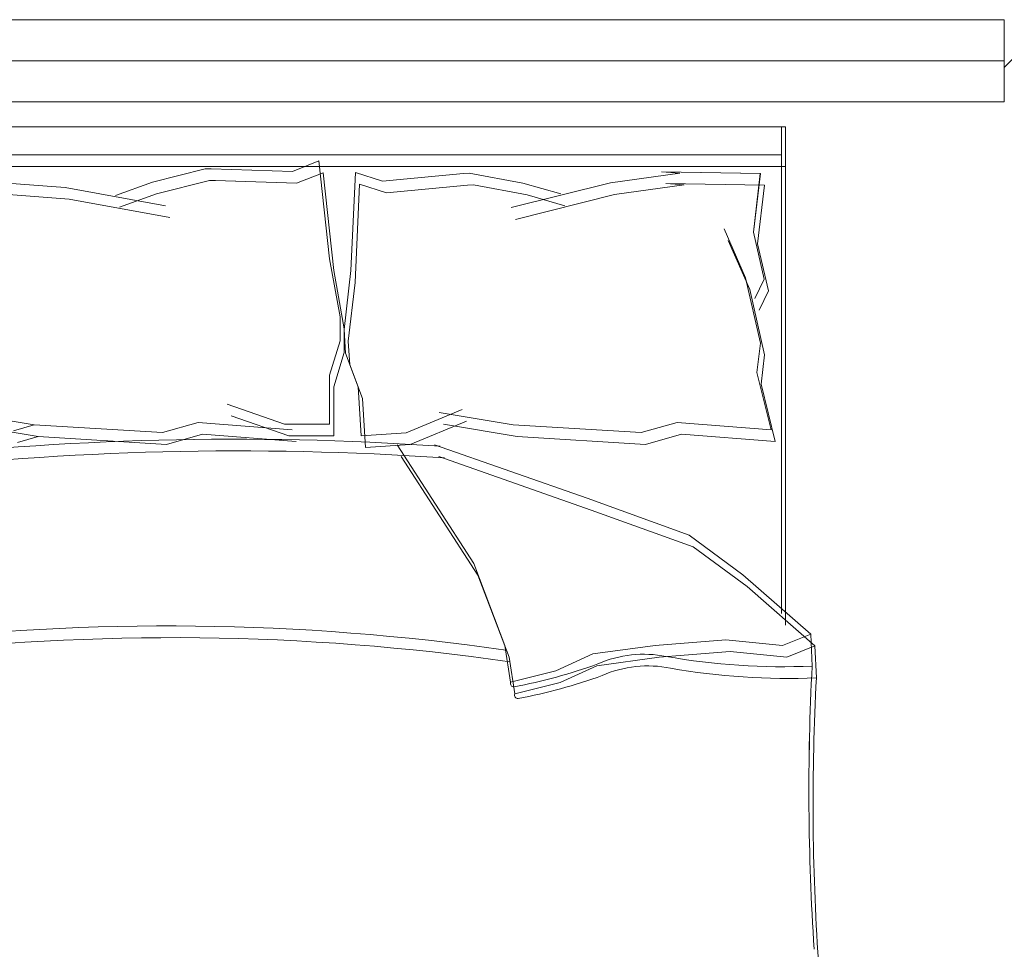
# Model space of a CAD drawing. Units: inches. Extents: x 1885 to 2748, y 783 to 2421.
# Tile 99 of 117: x 2395 to 2449, y 2302 to 2353. Entities that reach past the tile are written whole.
import ezdxf

# ---------------------------------------------------------------- set-up
doc = ezdxf.new("R2010")
doc.units = ezdxf.units.IN
doc.layers.add('A-FURN', color=8, linetype='Continuous', lineweight=13)
doc.layers.add('A-GLAZ', color=181, linetype='Continuous', lineweight=18)
doc.layers.add('A-WALL-PATT', color=85, linetype='Continuous', lineweight=13, true_color=0x58ba48)

# ---------------------------------------------------------------- blocks, each defined once
blk = doc.blocks.new('BED-DOUBLE')
for p, q in [((27.749, 52.866), (24.499, 49.161)), ((27.75, 52.866), (24.499, 49.161)), ((28.389, 53.095), (25.139, 49.389)), ((28.389, 53.094), (25.139, 49.389)), ((29.494, 52.946), (27.749, 52.866, 3.871)), ((28.369, 51.329), (27.749, 52.866)), ((29.494, 52.945), (27.75, 52.866, 3.871)), ((28.369, 51.329), (27.75, 52.866)), ((30.133, 53.174), (28.389, 53.095, 3.871)), ((30.133, 53.174), (28.389, 53.094, 3.871)), ((29.008, 51.558), (28.389, 53.095)), ((29.008, 51.557), (28.389, 53.094)), ((0.004, 51.493), (0.643, 51.492)), ((0.004, 3.474), (0.004, 51.493)), ((0.004, 51.264), (26.614, 51.264)), ((0.004, 51.264), (26.614, 51.264)), ((0.643, 51.493), (27.253, 51.493)), ((0.643, 51.492), (27.253, 51.492)), ((1.537, 3.474), (1.537, 51.264)), ((1.537, 3.474), (1.537, 51.264)), ((2.177, 3.702), (2.177, 51.493)), ((2.177, 3.702), (2.177, 51.492)), ((28.059, 48.232), (28.369, 51.329)), ((28.059, 48.231), (28.369, 51.329)), ((28.698, 48.46), (29.008, 51.558)), ((28.698, 48.46), (29.008, 51.557)), ((16.576, 50.697), (13.438, 49.922)), ((16.576, 50.697), (13.438, 49.921)), ((17.216, 50.925), (14.077, 50.15)), ((17.216, 50.925), (14.077, 50.15)), ((16.173, 45.565), (16.576, 50.697)), ((16.173, 45.565), (16.576, 50.697)), ((16.812, 45.794), (17.216, 50.925)), ((16.812, 45.793), (17.216, 50.925)), ((2.561, 50.111), (2.464, 44.708)), ((2.561, 50.11), (2.464, 44.708)), ((2.561, 50.111), (5.771, 49.732)), ((2.561, 50.11), (5.771, 49.732)), ((3.2, 50.339), (3.103, 44.937)), ((3.2, 50.339), (3.103, 44.936)), ((3.2, 50.339), (6.411, 49.96)), ((3.2, 50.339), (6.411, 49.96)), ((5.771, 49.732), (8.342, 50.327)), ((5.771, 49.732), (8.342, 50.327)), ((6.411, 49.96), (8.981, 50.556)), ((6.411, 49.96), (8.981, 50.555)), ((11.832, 50.111), (8.261, 49.308)), ((11.832, 50.111), (8.261, 49.308)), ((8.342, 50.327), (9.388, 49.813)), ((8.342, 50.327), (9.388, 49.813)), ((12.472, 50.339), (8.9, 49.537)), ((12.472, 50.339), (8.9, 49.536)), ((8.981, 50.556), (10.027, 50.042)), ((8.981, 50.555), (10.027, 50.041)), ((13.438, 49.922), (11.832, 50.111)), ((13.438, 49.921), (11.832, 50.111)), ((14.077, 50.15), (12.472, 50.339)), ((14.077, 50.15), (12.472, 50.339)), ((8.9, 49.537), (6.221, 48.355)), ((8.9, 49.536), (6.221, 48.355)), ((8.261, 49.308), (5.582, 48.127)), ((8.261, 49.308), (5.582, 48.127)), ((24.499, 49.161), (22.332, 46.218)), ((24.499, 49.161), (22.332, 46.218)), ((25.139, 49.389), (22.972, 46.447)), ((25.139, 49.389), (22.972, 46.447)), ((29.008, 44.588), (28.698, 48.46)), ((29.008, 44.588), (28.698, 48.46)), ((28.369, 44.36), (28.059, 48.232)), ((28.369, 44.36), (28.059, 48.231)), ((22.972, 46.447), (20.96, 40.871)), ((22.972, 46.447), (20.96, 40.871)), ((3.103, 44.937), (3.185, 45.939)), ((3.103, 44.936), (3.185, 45.939)), ((3.185, 45.939), (3.712, 42.141)), ((3.185, 45.939), (3.712, 42.141)), ((17.369, 43.833), (16.812, 45.794)), ((17.369, 43.833), (16.812, 45.793)), ((22.332, 46.218), (20.32, 40.643)), ((22.332, 46.218), (20.32, 40.643)), ((2.464, 44.708), (2.546, 45.711)), ((2.464, 44.708), (2.546, 45.711)), ((2.546, 45.711), (3.073, 41.913)), ((2.546, 45.711), (3.073, 41.913)), ((16.73, 43.605), (16.173, 45.565)), ((16.73, 43.605), (16.173, 45.565)), ((28.833, 40.953), (28.369, 44.36)), ((28.833, 40.952), (28.369, 44.36)), ((29.472, 41.181), (29.008, 44.588)), ((29.472, 41.181), (29.008, 44.588)), ((16.299, 36.595), (16.73, 43.605)), ((16.299, 36.595), (16.73, 43.605)), ((16.938, 36.823), (17.369, 43.833)), ((16.938, 36.823), (17.369, 43.833)), ((3.712, 42.141), (5.065, 36.722)), ((3.712, 42.141), (5.065, 36.722)), ((3.073, 41.913), (4.426, 36.494)), ((3.073, 41.913), (4.426, 36.493)), ((29.762, 38.939), (28.833, 40.953)), ((29.762, 38.939), (28.833, 40.952)), ((30.401, 39.168), (29.472, 41.181)), ((30.401, 39.167), (29.472, 41.181)), ((20.32, 40.643), (17.387, 32.305)), ((20.32, 40.643), (17.387, 32.305)), ((20.96, 40.871), (18.026, 32.533)), ((20.96, 40.871), (18.026, 32.533)), ((4.317, 39.427), (3.721, 37.362)), ((4.317, 39.427), (3.721, 37.362)), ((3.677, 39.199), (3.082, 37.134)), ((3.677, 39.199), (3.082, 37.134)), ((30.381, 36.461), (29.762, 38.939)), ((30.381, 36.461), (29.762, 38.939)), ((31.02, 36.69), (30.401, 39.168)), ((31.02, 36.689), (30.401, 39.167)), ((3.721, 37.362), (3.18, 34.432)), ((3.721, 37.362), (3.18, 34.431)), ((3.082, 37.134), (2.541, 34.203)), ((3.082, 37.134), (2.541, 34.203)), ((16.271, 32.791), (16.938, 36.823)), ((16.272, 32.791), (16.938, 36.823)), ((29.008, 36.38), (31.02, 36.69)), ((29.008, 36.38), (31.02, 36.689)), ((15.632, 32.563), (16.299, 36.595)), ((15.632, 32.563), (16.299, 36.595)), ((23.88, 34.448), (28.369, 36.152)), ((23.88, 34.448), (28.369, 36.151)), ((24.519, 34.676), (29.008, 36.38)), ((24.519, 34.676), (29.008, 36.38)), ((28.369, 36.152), (30.381, 36.461)), ((28.369, 36.151), (30.381, 36.461)), ((17.387, 30.258), (23.88, 34.448)), ((17.387, 30.258), (23.88, 34.448)), ((18.026, 30.486), (24.519, 34.676)), ((18.026, 30.486), (24.519, 34.676)), ((2.541, 34.203), (2.561, 33.882)), ((2.541, 34.203), (2.561, 33.882)), ((3.18, 34.432), (3.2, 34.111)), ((3.18, 34.431), (3.2, 34.11)), ((3.2, 34.111), (3.622, 29.683)), ((3.2, 34.11), (3.622, 29.683)), ((17.382, 30.977), (16.097, 34.048)), ((17.382, 30.977), (16.097, 34.048)), ((2.561, 33.882), (2.982, 29.454)), ((2.561, 33.882), (2.982, 29.454)), ((16.743, 30.749), (15.458, 33.819)), ((16.743, 30.749), (15.458, 33.819)), ((16.896, 28.296), (16.743, 30.749)), ((16.896, 28.296), (16.743, 30.749)), ((17.536, 28.525), (17.382, 30.977)), ((17.536, 28.524), (17.382, 30.977)), ((3.622, 29.683), (3.135, 28.204)), ((3.622, 29.683), (3.135, 28.204)), ((2.982, 29.454), (2.495, 27.976)), ((2.982, 29.454), (2.495, 27.975)), ((3.135, 28.204), (8.51, 27.961)), ((3.135, 28.204), (8.51, 27.96)), ((12.38, 27.435), (14.22, 28.129)), ((12.38, 27.434), (14.22, 28.129)), ((13.02, 27.663), (14.86, 28.357)), ((13.02, 27.663), (14.86, 28.357)), ((14.22, 28.129), (16.896, 28.296)), ((14.22, 28.129), (16.896, 28.296)), ((14.86, 28.357), (17.536, 28.525)), ((14.86, 28.357), (17.536, 28.524)), ((2.495, 27.976), (7.871, 27.732)), ((2.495, 27.975), (7.871, 27.732)), ((7.871, 27.732), (11.082, 27.354)), ((7.871, 27.732), (11.082, 27.353)), ((8.51, 27.961), (11.721, 27.582)), ((8.51, 27.96), (11.721, 27.582)), ((11.721, 27.582), (13.02, 27.663)), ((11.721, 27.582), (13.02, 27.663)), ((7.224, 26.56), (10.404, 27.138)), ((7.224, 26.559), (10.405, 27.137)), ((7.863, 26.788), (11.044, 27.366)), ((7.863, 26.788), (11.044, 27.366)), ((10.404, 27.138), (11.706, 27.138)), ((10.405, 27.137), (11.706, 27.137)), ((11.044, 27.366), (12.345, 27.366)), ((11.044, 27.366), (12.345, 27.366)), ((11.082, 27.354), (12.38, 27.435)), ((11.082, 27.353), (12.38, 27.434)), ((11.706, 27.138), (13.585, 26.56)), ((11.706, 27.137), (13.585, 26.559)), ((12.345, 27.366), (14.225, 26.788)), ((12.345, 27.366), (14.225, 26.788)), ((1.874, 25.981), (7.224, 26.56)), ((1.874, 25.981), (7.224, 26.559)), ((2.513, 26.21), (7.863, 26.788)), ((2.513, 26.209), (7.863, 26.788)), ((13.585, 26.56), (16.267, 26.56)), ((13.585, 26.559), (16.267, 26.559)), ((14.225, 26.788), (16.906, 26.788)), ((14.225, 26.788), (16.906, 26.788)), ((16.267, 26.56), (16.267, 24.102)), ((16.267, 26.559), (16.267, 24.102)), ((16.906, 26.788), (16.906, 24.33)), ((16.906, 26.788), (16.906, 24.33)), ((2.452, 24.536), (1.874, 25.981)), ((2.452, 24.535), (1.874, 25.981)), ((3.091, 24.764), (2.513, 26.21)), ((3.091, 24.764), (2.513, 26.209)), ((2.947, 20.319), (3.091, 24.764)), ((2.947, 20.318), (3.091, 24.764)), ((2.308, 20.09), (2.452, 24.536)), ((2.308, 20.09), (2.452, 24.535)), ((16.906, 24.33), (15.815, 21.186)), ((16.906, 24.33), (15.815, 21.186)), ((16.173, 19.383), (16.576, 24.515)), ((16.173, 19.382), (16.576, 24.514)), ((16.812, 19.611), (17.216, 24.743)), ((16.812, 19.611), (17.216, 24.743)), ((16.267, 24.102), (15.176, 20.957)), ((16.267, 24.102), (15.176, 20.957)), ((2.308, 19.769), (2.308, 20.09)), ((2.308, 19.768), (2.308, 20.09)), ((2.947, 19.997), (2.947, 20.319)), ((2.947, 19.997), (2.947, 20.318)), ((3.67, 17.106), (2.947, 19.997)), ((3.67, 17.105), (2.947, 19.997)), ((3.031, 16.877), (2.308, 19.769)), ((3.031, 16.877), (2.308, 19.768)), ((16.73, 17.422), (16.173, 19.383)), ((16.73, 17.422), (16.173, 19.382)), ((17.369, 17.651), (16.812, 19.611)), ((17.369, 17.65), (16.812, 19.611)), ((3.959, 12.335), (4.971, 17.829)), ((3.959, 12.335), (4.971, 17.828)), ((3.32, 12.107), (4.332, 17.6)), ((3.32, 12.107), (4.332, 17.6)), ((16.299, 10.412), (16.73, 17.422)), ((16.299, 10.412), (16.73, 17.422)), ((16.938, 10.641), (17.369, 17.651)), ((16.938, 10.64), (17.369, 17.65)), ((3.753, 14.854), (3.031, 16.877)), ((3.753, 14.853), (3.031, 16.877)), ((4.393, 15.082), (3.67, 17.106)), ((4.393, 15.082), (3.67, 17.105)), ((3.031, 8.284), (3.32, 12.107)), ((3.031, 8.283), (3.32, 12.107)), ((3.67, 8.512), (3.959, 12.335)), ((3.67, 8.512), (3.959, 12.335)), ((15.632, 6.38), (16.299, 10.412)), ((15.632, 6.38), (16.299, 10.412)), ((16.271, 6.609), (16.938, 10.641)), ((16.272, 6.609), (16.938, 10.64)), ((16.299, 10.412), (16.622, 9.279)), ((16.299, 10.412), (16.622, 9.279)), ((16.938, 10.641), (17.261, 9.508)), ((16.938, 10.64), (17.261, 9.507))]:
    blk.add_line(p, q)
for centre, radius, start, end in [((-6.653, 51.326), 36.183, 349.8763, 2.5657), ((-6.653, 51.326), 36.183, 349.8763, 2.5657), ((36.319, 182.265), 129.499, 266.97912, 273.83645), ((36.319, 182.264), 129.499, 266.97912, 273.83645), ((-6.013, 51.554), 36.183, 349.8763, 2.5657), ((-6.013, 51.554), 36.183, 349.8763, 2.5657), ((36.958, 182.493), 129.499, 266.97912, 273.83645), ((36.958, 182.493), 129.499, 266.97912, 273.83645), ((35.07, 43.742), 6.224, 168.6608, 203.7384), ((35.07, 43.742), 6.224, 168.6608, 203.7384), ((35.709, 43.971), 6.224, 168.6608, 203.7384), ((35.709, 43.97), 6.224, 168.6608, 203.7384), ((2.125, 31.381), 29.654, 10.6617, 19.8806), ((2.125, 31.381), 29.654, 10.6617, 19.8806), ((1.486, 31.152), 29.654, 10.6617, 19.8806), ((1.486, 31.152), 29.654, 10.6617, 19.8806), ((30.443, 36.635), 0.185, 250.2464, 1.1377), ((30.443, 36.635), 0.185, 250.2464, 1.1377), ((31.082, 36.863), 0.185, 250.2464, 1.1377), ((31.082, 36.863), 0.185, 250.2464, 1.1377), ((156.32, 17.754), 129.02, 171.78449, 186.90062), ((156.32, 17.754), 129.02, 171.78449, 186.90062), ((156.959, 17.983), 129.02, 171.78449, 186.90062), ((156.959, 17.983), 129.02, 171.78449, 186.90062), ((182.695, 21.586), 164.969, 176.08655, 186.78213), ((182.695, 21.586), 164.969, 176.08655, 186.78213), ((182.056, 21.358), 164.969, 176.08655, 186.78213), ((182.056, 21.357), 164.969, 176.08655, 186.78213)]:
    blk.add_arc(centre, radius, start, end)
blk = doc.blocks.new('WIN-60')
for p, q in [((0.004, 59.998), (4.504, 59.998)), ((0.004, 59.998), (0.004, -0.002)), ((4.504, 59.998), (2.254, 59.998)), ((2.254, 59.998), (2.254, -0.002)), ((4.504, -0.002), (4.504, 59.998))]:
    blk.add_line(p, q)

msp = doc.modelspace()

# ---------------------------------------------------------------- hatches: boundary and pattern name
at = {"layer": 'A-WALL-PATT'}
h = msp.add_hatch(dxfattribs=at)
h.set_pattern_fill('ANSI32', color=256)
h.paths.add_polyline_path([(2007.772, 2318.006), (1980.774, 2318.006), (1980.774, 2281.215), (1985.274, 2281.215), (1985.274, 2313.506), (2007.772, 2313.506), (2007.772, 2315.756)])
h.paths.add_polyline_path([(2094.324, 2318.006), (2067.772, 2318.006), (2067.772, 2313.506), (2094.324, 2313.506), (2094.324, 2315.756)])
h.paths.add_polyline_path([(2131.367, 2315.756), (2131.367, 2318.006), (2131.189, 2318.006), (2112.609, 2318.006), (2112.609, 2313.506), (2117.274, 2313.506), (2117.274, 2255.201), (2121.774, 2255.201), (2121.774, 2313.506), (2131.367, 2313.506)])
h.paths.add_polyline_path([(2190.512, 2318.006), (2155.367, 2318.006), (2155.367, 2313.506), (2169.774, 2313.506), (2169.774, 2229.506), (2121.774, 2229.506), (2121.774, 2233.451), (2119.524, 2233.451), (2117.274, 2233.451), (2117.274, 2201.101), (2121.774, 2201.101), (2121.774, 2225.006), (2169.774, 2225.006), (2169.774, 2165.006), (2306.274, 2165.006), (2306.274, 2066.006), (2310.774, 2066.006), (2344.274, 2066.006), (2486.274, 2066.006), (2486.274, 1886.006), (2483.02, 1886.006), (2483.02, 1881.506), (2486.274, 1881.506), (2486.274, 1880.678), (2490.774, 1880.678), (2490.774, 2070.506), (2344.274, 2070.506), (2310.774, 2070.506), (2310.774, 2165.006), (2310.774, 2173.636), (2308.524, 2173.636), (2306.274, 2173.636), (2306.274, 2169.506), (2174.274, 2169.506), (2174.274, 2313.506), (2190.512, 2313.506), (2190.512, 2315.756)])
h.paths.add_polyline_path([(1985.274, 2221.215), (1980.774, 2221.215), (1980.774, 2165.006), (1992.774, 2165.006), (1992.774, 2141.927), (1997.274, 2141.927), (1997.274, 2165.006), (2117.274, 2165.006), (2117.274, 2163.126), (2121.774, 2163.126), (2121.774, 2172.734), (2119.524, 2172.734), (2117.274, 2172.734), (2117.274, 2169.506), (1985.274, 2169.506)])
h.paths.add_polyline_path([(1997.274, 2105.927), (1992.774, 2105.927), (1992.774, 2070.506), (2016.774, 2070.506), (2016.774, 2059.123), (2019.024, 2059.123), (2021.274, 2059.123), (2021.274, 2070.506), (2117.274, 2070.506), (2117.274, 2022.506), (2114.423, 2022.506), (2114.423, 2018.006), (2123.627, 2018.006), (2123.627, 2020.256), (2123.627, 2022.506), (2121.774, 2022.506), (2121.774, 2142.587), (2119.524, 2142.587), (2117.274, 2142.587), (2117.274, 2075.006), (1997.274, 2075.006)])
h.paths.add_polyline_path([(2092.029, 2020.256), (2092.029, 2022.506), (2021.274, 2022.506), (2021.274, 2035.123), (2016.774, 2035.123), (2016.774, 2018.006), (2016.774, 1978.784), (2021.274, 1978.784), (2021.274, 2018.006), (2092.029, 2018.006)])
h.paths.add_polyline_path([(2260.938, 2022.506), (2153.105, 2022.506), (2153.105, 2020.256), (2153.105, 2018.006), (2155.274, 2018.006), (2155.274, 1886.006), (2107.629, 1886.006), (2107.629, 1881.506), (2182.911, 1881.506), (2182.911, 1883.756), (2182.911, 1886.006), (2159.774, 1886.006), (2159.774, 2018.006), (2260.938, 2018.006), (2260.938, 2020.256)])
h.paths.add_polyline_path([(2047.629, 1883.756), (2047.629, 1886.006), (2021.274, 1886.006), (2021.274, 1918.784), (2019.024, 1918.784), (2016.774, 1918.784), (2016.774, 1881.506), (2047.629, 1881.506)])
h.paths.add_polyline_path([(2306.361, 1883.756), (2306.361, 1886.006), (2296.274, 1886.006), (2296.274, 1982.006), (2316.535, 1982.006), (2316.535, 1984.256), (2316.535, 1986.506), (2296.274, 1986.506), (2296.274, 2022.506), (2289.276, 2022.506), (2289.276, 2018.006), (2291.774, 2018.006), (2291.774, 1886.006), (2242.911, 1886.006), (2242.911, 1881.506), (2306.361, 1881.506)], flags=17)
h.paths.add_polyline_path([(1985.274, 1843.006), (2021.6, 1843.006), (2021.534, 1845.441), (2021.477, 1847.506), (1980.774, 1847.506), (1980.774, 1809.446), (1985.274, 1809.446)])
h.paths.add_polyline_path([(2131.482, 1845.256), (2131.482, 1847.506), (2081.534, 1847.506), (2081.534, 1843.006), (2117.274, 1843.006), (2117.274, 1784.147), (2119.524, 1784.147), (2121.774, 1784.147), (2121.774, 1843.006), (2131.482, 1843.006)])
h.paths.add_polyline_path([(2203.886, 1847.506), (2155.482, 1847.506), (2155.482, 1843.006), (2169.774, 1843.006), (2169.774, 1759.006), (2121.774, 1759.006), (2121.774, 1761.457), (2117.274, 1761.457), (2117.274, 1730.429), (2121.774, 1730.429), (2121.774, 1754.506), (2177.421, 1754.506), (2177.421, 1756.756), (2177.421, 1759.006), (2174.274, 1759.006), (2174.274, 1843.006), (2203.886, 1843.006)])
h.paths.add_polyline_path([(2335.554, 1845.256), (2335.554, 1847.506), (2239.886, 1847.506), (2239.886, 1843.006), (2306.274, 1843.006), (2306.274, 1759.006), (2199.486, 1759.006), (2199.486, 1754.506), (2310.774, 1754.506), (2310.774, 1843.006), (2335.554, 1843.006)])
h.paths.add_polyline_path([(2348.774, 2022.506), (2344.274, 2022.506), (2344.274, 1986.506), (2341.681, 1986.506), (2341.681, 1982.006), (2344.274, 1982.006), (2344.274, 1886.006), (2330.361, 1886.006), (2330.361, 1881.506), (2361.627, 1881.506), (2361.627, 1883.756), (2361.627, 1886.006), (2348.774, 1886.006)], flags=17)
h.paths.add_polyline_path([(2283.251, 2315.756), (2283.251, 2318.006), (2238.512, 2318.006), (2238.512, 2313.506), (2283.251, 2313.506)], flags=17)
h.paths.add_polyline_path([(2363.274, 2348.006), (2388.677, 2348.006), (2388.677, 2350.256), (2388.677, 2352.506), (2358.774, 2352.506), (2358.774, 2348.006), (2358.774, 2318.006), (2344.481, 2318.006), (2344.481, 2313.506), (2358.774, 2313.506), (2358.774, 2229.506), (2310.774, 2229.506), (2310.774, 2231.952), (2306.274, 2231.952), (2306.274, 2205.611), (2310.774, 2205.611), (2310.774, 2225.006), (2358.774, 2225.006), (2358.774, 2211.506), (2452.329, 2211.506), (2452.329, 2213.756), (2452.329, 2216.006), (2363.274, 2216.006), (2363.274, 2318.006)])
h.paths.add_polyline_path([(2310.774, 2313.506), (2320.481, 2313.506), (2320.481, 2315.756), (2320.481, 2318.006), (2302.728, 2318.006), (2302.728, 2313.506), (2306.274, 2313.506), (2306.274, 2251.076), (2310.774, 2251.076)], flags=17)
h.paths.add_polyline_path([(2490.774, 2352.506), (2486.274, 2352.506), (2448.677, 2352.506), (2448.677, 2348.006), (2486.274, 2348.006), (2486.274, 2318.006), (2486.274, 2216.006), (2481.78, 2216.006), (2481.78, 2211.506), (2486.274, 2211.506), (2486.274, 2165.006), (2493.289, 2165.006), (2493.289, 2167.256), (2493.289, 2169.506), (2490.774, 2169.506), (2490.774, 2313.506), (2494.429, 2313.506), (2494.429, 2318.006), (2490.774, 2318.006)])
h.paths.add_polyline_path([(2534.653, 2318.006), (2515.691, 2318.006), (2515.691, 2313.506), (2534.653, 2313.506), (2534.653, 2315.756)])
h.paths.add_polyline_path([(2618.274, 2318.006), (2594.653, 2318.006), (2594.653, 2313.506), (2613.774, 2313.506), (2613.774, 2281.706), (2618.274, 2281.706)])
h.paths.add_polyline_path([(2618.274, 2221.706), (2613.774, 2221.706), (2613.774, 2169.506), (2554.019, 2169.506), (2554.019, 2165.006), (2613.774, 2165.006), (2613.774, 2152.878), (2618.274, 2152.878)])
h.paths.add_polyline_path([(2618.274, 2128.878), (2616.024, 2128.878), (2613.774, 2128.878), (2613.774, 2117.006), (2529.774, 2117.006), (2529.774, 2165.006), (2532.848, 2165.006), (2532.848, 2169.506), (2522.867, 2169.506), (2522.867, 2165.006), (2525.274, 2165.006), (2525.274, 2117.006), (2525.274, 2112.506), (2525.274, 2108.576), (2529.774, 2108.576), (2529.774, 2112.506), (2613.774, 2112.506), (2613.774, 2080.19), (2618.274, 2080.19)])
h.paths.add_polyline_path([(2618.274, 2044.19), (2616.024, 2044.19), (2613.774, 2044.19), (2613.774, 2015.506), (2529.774, 2015.506), (2529.774, 2088.582), (2527.524, 2088.582), (2525.274, 2088.582), (2525.274, 2011.006), (2613.774, 2011.006), (2613.774, 1956.755), (2618.274, 1956.755)])
h.paths.add_polyline_path([(2618.274, 1881.506), (2618.274, 1896.755), (2613.774, 1896.755), (2613.774, 1881.506), (2613.774, 1847.506), (2592.715, 1847.506), (2592.715, 1843.006), (2613.774, 1843.006), (2613.774, 1765.006), (2613.774, 1760.506), (2609.621, 1760.506), (2609.621, 1756.006), (2613.774, 1756.006), (2613.774, 1660.006), (2608.544, 1660.006), (2608.544, 1655.506), (2613.774, 1655.506), (2613.774, 1508.158), (2618.274, 1508.158)])
h.paths.add_polyline_path([(2565.774, 1843.006), (2568.997, 1843.006), (2568.997, 1847.506), (2490.774, 1847.506), (2490.774, 1849.7), (2488.524, 1849.7), (2486.274, 1849.7), (2486.274, 1847.506), (2477.274, 1847.506), (2477.274, 1838.506), (2477.274, 1821.493), (2486.274, 1821.493), (2486.274, 1838.506), (2561.274, 1838.506), (2561.274, 1765.006), (2486.274, 1765.006), (2486.274, 1786.157), (2477.274, 1786.157), (2477.274, 1765.006), (2477.274, 1756.006), (2486.274, 1756.006), (2565.774, 1756.006), (2585.621, 1756.006), (2585.621, 1758.256), (2585.621, 1760.506), (2565.774, 1760.506), (2565.774, 1765.006)])
h.paths.add_polyline_path([(2486.274, 1651.006), (2561.274, 1651.006), (2561.274, 1567.006), (2486.274, 1567.006), (2486.274, 1591.321), (2477.274, 1591.321), (2477.274, 1567.006), (2477.274, 1558.006), (2477.274, 1555.439), (2481.774, 1555.439), (2481.774, 1558.006), (2568.653, 1558.006), (2568.653, 1560.256), (2568.653, 1562.506), (2565.774, 1562.506), (2565.774, 1655.506), (2584.544, 1655.506), (2584.544, 1657.756), (2584.544, 1660.006), (2565.774, 1660.006), (2486.274, 1660.006), (2477.274, 1660.006), (2477.274, 1651.006), (2477.274, 1632.989), (2486.274, 1632.989)])
h.paths.add_polyline_path([(2449.967, 1883.756), (2449.967, 1886.006), (2421.627, 1886.006), (2421.627, 1881.506), (2449.967, 1881.506)], flags=17)
h.paths.add_polyline_path([(2447.274, 1847.506), (2395.554, 1847.506), (2395.554, 1843.006), (2442.774, 1843.006), (2442.774, 1809.27), (2447.274, 1809.27)])
h.paths.add_polyline_path([(1985.274, 1749.446), (1980.774, 1749.446), (1980.774, 1694.504), (1985.274, 1694.504), (1985.274, 1694.506), (1986.897, 1694.506), (1986.897, 1697.78), (1986.897, 1699.006), (1985.274, 1699.006)])
h.paths.add_polyline_path([(2152.774, 1699.006), (2121.774, 1699.006), (2121.774, 1703.668), (2119.524, 1703.668), (2117.274, 1703.668), (2117.274, 1699.006), (2009.219, 1699.006), (2009.219, 1694.506), (2148.274, 1694.506), (2148.274, 1692.631), (2152.774, 1692.631)])
h.paths.add_polyline_path([(2016.274, 1694.506), (2011.774, 1694.506), (2011.774, 1558.006), (2040.806, 1558.006), (2040.806, 1560.256), (2040.806, 1562.506), (2016.274, 1562.506)])
h.paths.add_polyline_path([(2152.774, 1663.017), (2150.524, 1663.017), (2148.274, 1663.017), (2148.274, 1562.506), (2100.806, 1562.506), (2100.806, 1558.006), (2165.119, 1558.006), (2165.119, 1560.256), (2165.119, 1562.506), (2152.774, 1562.506), (2152.774, 1610.506), (2224.774, 1610.506), (2224.774, 1607.99), (2229.274, 1607.99), (2229.274, 1615.006), (2152.774, 1615.006)])
h.paths.add_polyline_path([(2238.613, 1560.256), (2238.613, 1562.506), (2229.274, 1562.506), (2229.274, 1588.756), (2227.024, 1588.763), (2224.774, 1588.771), (2224.774, 1562.506), (2189.119, 1562.506), (2189.119, 1558.006), (2238.613, 1558.006)])
h.paths.add_polyline_path([(2336.024, 1560.256), (2336.024, 1562.506), (2310.774, 1562.506), (2310.774, 1656.347), (2308.524, 1656.347), (2306.274, 1656.347), (2306.274, 1562.506), (2286.613, 1562.506), (2286.613, 1558.006), (2336.024, 1558.006)])
h.paths.add_polyline_path([(2447.274, 1690.968), (2445.024, 1690.968), (2442.774, 1690.968), (2442.774, 1687.006), (2306.274, 1687.006), (2306.274, 1680.75), (2310.774, 1680.75), (2310.774, 1682.506), (2442.774, 1682.506), (2442.774, 1562.506), (2396.024, 1562.506), (2396.024, 1558.006), (2447.274, 1558.006)])
h.paths.add_polyline_path([(2447.274, 1749.27), (2445.024, 1749.27), (2442.774, 1749.27), (2442.774, 1717.232), (2447.274, 1717.232)])
h.paths.add_polyline_path([(2044.674, 1521.756), (2044.674, 1524.006), (2007.274, 1524.006), (2007.274, 1503.49), (2009.524, 1503.49), (2011.774, 1503.49), (2011.774, 1519.506), (2044.674, 1519.506)])
h.paths.add_polyline_path([(2177.969, 1521.756), (2177.969, 1524.006), (2104.674, 1524.006), (2104.674, 1519.506), (2145.774, 1519.506), (2145.774, 1387.506), (2143.37, 1387.506), (2143.37, 1383.006), (2251.585, 1383.006), (2251.585, 1385.256), (2251.585, 1387.506), (2150.274, 1387.506), (2150.274, 1519.506), (2177.969, 1519.506)])
h.paths.add_polyline_path([(2298.704, 1524.006), (2237.969, 1524.006), (2237.969, 1519.506), (2282.274, 1519.506), (2282.274, 1387.506), (2279.683, 1387.506), (2279.683, 1383.006), (2286.774, 1383.006), (2286.774, 1419.006), (2312.451, 1419.006), (2312.451, 1421.256), (2312.451, 1423.506), (2286.774, 1423.506), (2286.774, 1519.506), (2298.704, 1519.506), (2298.704, 1521.722)], flags=17)
h.paths.add_polyline_path([(2361.897, 1521.756), (2361.897, 1524.006), (2322.704, 1524.006), (2322.704, 1519.506), (2334.774, 1519.506), (2334.774, 1423.506), (2331.93, 1423.506), (2331.93, 1419.006), (2334.774, 1419.006), (2334.774, 1387.506), (2334.774, 1383.228), (2339.274, 1383.228), (2339.274, 1387.506), (2339.274, 1519.506), (2361.897, 1519.506)], flags=17)
h.paths.add_polyline_path([(2447.274, 1521.756), (2447.274, 1524.006), (2421.897, 1524.006), (2421.897, 1519.506), (2447.274, 1519.506)], flags=17)
h.paths.add_polyline_path([(2481.774, 1529.6), (2479.524, 1529.6), (2477.274, 1529.6), (2477.274, 1524.006), (2474.489, 1524.006), (2474.489, 1519.506), (2477.274, 1519.506), (2477.274, 1334.506), (2296.774, 1334.506), (2296.774, 1240.506), (2160.274, 1240.506), (2160.274, 1180.506), (2112.274, 1180.506), (2112.274, 1207.692), (2110.024, 1207.692), (2107.774, 1207.692), (2107.774, 1171.609), (2112.274, 1171.609), (2112.274, 1176.006), (2160.274, 1176.006), (2160.274, 1092.006), (2144.221, 1092.006), (2144.221, 1087.506), (2189.497, 1087.506), (2189.497, 1089.756), (2189.497, 1092.006), (2164.774, 1092.006), (2164.774, 1236.006), (2296.774, 1236.006), (2296.774, 1231.912), (2301.274, 1231.912), (2301.274, 1330.006), (2481.774, 1330.006), (2481.774, 1387.506)])
h.paths.add_polyline_path([(2618.274, 1448.158), (2613.774, 1448.158), (2613.774, 1382.506), (2529.774, 1382.506), (2525.274, 1382.506), (2525.274, 1307.062), (2529.774, 1307.062), (2529.774, 1378.006), (2613.774, 1378.006), (2613.774, 1354.988), (2618.274, 1354.988)])
h.paths.add_polyline_path([(2618.274, 1318.988), (2613.774, 1318.988), (2613.774, 1281.006), (2529.774, 1281.006), (2529.774, 1283.786), (2527.524, 1283.786), (2525.274, 1283.786), (2525.274, 1228.506), (2516.794, 1228.506), (2516.794, 1224.006), (2533.484, 1224.006), (2533.484, 1226.256), (2533.484, 1228.506), (2529.774, 1228.506), (2529.774, 1276.506), (2613.774, 1276.506), (2613.774, 1266.02), (2618.274, 1266.02)])
h.paths.add_polyline_path([(2618.274, 1134.964), (2613.774, 1134.964), (2613.774, 1092.006), (2594.545, 1092.006), (2594.545, 1087.506), (2618.274, 1087.506)])
h.paths.add_polyline_path([(2534.545, 1092.006), (2509.765, 1092.006), (2509.765, 1087.506), (2534.545, 1087.506), (2534.545, 1089.756)])
h.paths.add_polyline_path([(2481.274, 1224.006), (2484.117, 1224.006), (2484.117, 1226.256), (2484.117, 1228.506), (2476.774, 1228.506), (2476.774, 1198.506), (2471.61, 1198.506), (2471.61, 1194.006), (2476.774, 1194.006), (2476.774, 1062.006), (2436.894, 1062.006), (2436.894, 1057.506), (2476.774, 1057.506), (2481.274, 1057.506), (2481.274, 1062.006), (2481.274, 1087.506), (2485.354, 1087.506), (2485.354, 1089.756), (2485.354, 1092.006), (2481.274, 1092.006), (2481.274, 1117.506)])
h.paths.add_polyline_path([(2439.898, 1198.506), (2349.274, 1198.506), (2349.274, 1194.006), (2349.274, 1180.506), (2301.274, 1180.506), (2301.274, 1201.896), (2299.024, 1201.896), (2296.774, 1201.896), (2296.774, 1172.335), (2299.024, 1172.335), (2301.274, 1172.335), (2301.274, 1176.006), (2349.274, 1176.006), (2349.274, 1092.006), (2334.452, 1092.006), (2334.452, 1087.506), (2349.274, 1087.506), (2349.274, 1057.506), (2353.774, 1057.506), (2376.894, 1057.506), (2376.894, 1059.756), (2376.894, 1062.006), (2353.774, 1062.006), (2353.774, 1087.506), (2353.774, 1180.506), (2353.774, 1194.006), (2439.898, 1194.006), (2439.898, 1196.256)])
h.paths.add_polyline_path([(2270.596, 1089.756), (2270.596, 1092.006), (2249.497, 1092.006), (2249.497, 1087.506), (2270.596, 1087.506)], flags=17)
h.paths.add_polyline_path([(2310.452, 1092.006), (2301.274, 1092.006), (2301.274, 1153.292), (2296.774, 1153.292), (2296.774, 1092.006), (2293.786, 1092.006), (2293.786, 1087.506), (2310.452, 1087.506), (2310.452, 1089.756)], flags=17)
h.paths.add_polyline_path([(2112.274, 1150.328), (2110.024, 1150.328), (2107.774, 1150.328), (2107.774, 1092.006), (2104.465, 1092.006), (2104.465, 1087.506), (2120.221, 1087.506), (2120.221, 1089.756), (2120.221, 1092.006), (2112.274, 1092.006)])
h.paths.add_polyline_path([(2082.172, 1092.006), (2058.144, 1092.006), (2058.144, 1087.506), (2082.172, 1087.506), (2082.172, 1089.756)])
h.paths.add_polyline_path([(1975.774, 1145.638), (1971.274, 1145.638), (1971.274, 1087.506), (1980.774, 1087.506), (1998.144, 1087.506), (1998.144, 1089.756), (1998.144, 1092.006), (1985.274, 1092.006), (1975.774, 1092.006)])
h.paths.add_polyline_path([(2112.274, 1244.385), (2110.024, 1244.385), (2107.774, 1244.385), (2107.774, 1240.506), (1992.274, 1240.506), (1992.274, 1271.008), (1987.774, 1271.008), (1987.774, 1240.506), (1980.774, 1240.506), (1975.774, 1240.506), (1971.274, 1240.506), (1971.274, 1205.638), (1975.774, 1205.638), (1975.774, 1236.006), (2107.774, 1236.006), (2107.774, 1233.444), (2112.274, 1233.444), (2112.274, 1236.006)])
h.paths.add_polyline_path([(2112.274, 1383.006), (2114.783, 1383.006), (2114.783, 1385.256), (2114.783, 1387.506), (2102.476, 1387.506), (2102.476, 1383.006), (2107.774, 1383.006), (2107.774, 1335.006), (2011.774, 1335.006), (2011.774, 1349.939), (2007.274, 1349.939), (2007.274, 1335.006), (1987.774, 1335.006), (1987.774, 1330.506), (1987.774, 1307.008), (1992.274, 1307.008), (1992.274, 1330.506), (2007.274, 1330.506), (2107.774, 1330.506), (2107.774, 1264.711), (2112.274, 1264.711)])
h.paths.add_polyline_path([(2077.857, 1387.506), (2011.774, 1387.506), (2011.774, 1390.036), (2009.524, 1390.036), (2007.274, 1390.036), (2007.274, 1373.939), (2011.774, 1373.939), (2011.774, 1383.006), (2077.857, 1383.006)])
h.paths.add_polyline_path([(2011.774, 1443.49), (2007.274, 1443.49), (2007.274, 1410.248), (2011.774, 1410.248)])

# ---------------------------------------------------------------- block references
at = {"layer": 'A-FURN', "rotation": 269.9999998331857}
msp.add_blockref('BED-DOUBLE', (2385.229, 2346.652), dxfattribs=at)
at = {"layer": 'A-GLAZ', "extrusion": (0, 0, -1), "zscale": -1, "rotation": 90}
msp.add_blockref('WIN-60', (-2388.679, 2348.002), dxfattribs=at)

doc.saveas('drawing.dxf')
